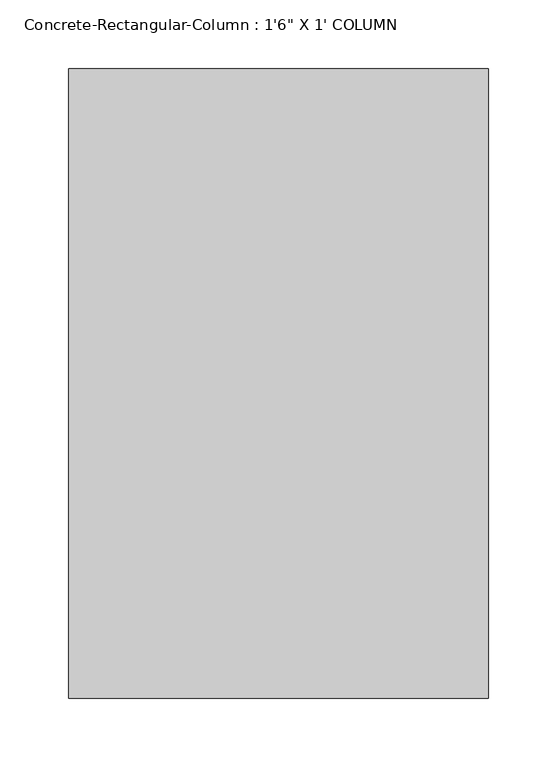
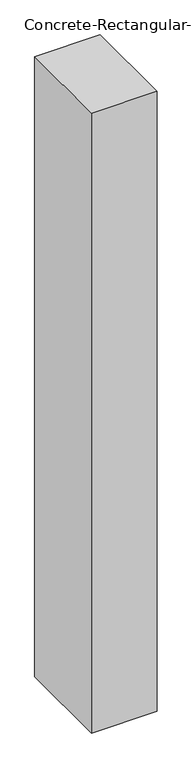
"""IFC4 building model written with IfcOpenShell, lengths in millimetres: column geometry."""

from ifc_helpers import new_model, si_unit, frame, origin, place, context, project, spatial, polyline, outline, extrude, source, transform, mapped, element, save


def column_6a931455(model_context):
    return source(origin(), model_context, "Body", "SweptSolid", [
        extrude(outline(polyline([(152.4, 228.6), (152.4, -228.6), (-152.4, -228.6), (-152.4, 228.6), (152.4, 228.6)])), frame((0.0, 0.0, 304.8), z_axis=(0.0, 0.0, 1.0), x_axis=(1.0, 0.0, 0.0)), (0.0, 0.0, 1.0), 3048.0),
    ])


if __name__ == "__main__":
    model = new_model("IFC4")
    model_context = context("Model", 3, world=origin())
    ifc_project = project(units=[si_unit("LENGTHUNIT", "METRE", prefix="MILLI")], contexts=[model_context])
    site = spatial("IfcSite", under=ifc_project)
    building = spatial("IfcBuilding", under=site)
    placement = place(None, origin())
    column_shape = column_6a931455(model_context)
    element("IfcColumn", 1, ObjectType="Concrete-Rectangular-Column : 1'6\" X 1' COLUMN", at=placement, inside=building, context=model_context, shape_type="MappedRepresentation", body=[
        mapped(column_shape, transform((0.0, 0.0, 0.0), x_axis=(1.0, 0.0, 0.0), y_axis=(0.0, 1.0, 0.0), z_axis=(0.0, 0.0, 1.0))),
    ])
    save(model, "model.ifc")

# Revit data of these elements
# Type "Concrete-Rectangular-Column : 1'6\" X 1' COLUMN"
#   Assembly Code = "B10"
#   b = 1' - 0"
#   h = 1' - 6"
#   Structural Material [instance default] = Concrete, Cast-in-Place gray
# Element 1 (IfcColumn, "Concrete-Rectangular-Column : 1'6\" X 1' COLUMN")
#   Structural Material = WARM BEIGE COLOUR
#   Materials on its faces: "WARM BEIGE COLOUR"
# Materials
#   "Concrete, Cast-in-Place gray": class "Concrete", colour RGB 192 192 192, transparency 0, Description = "Cast-in-place concrete", Cost = 0
#   "WARM BEIGE COLOUR": class "Generic", colour RGB 120 120 120, transparency 0, Cost = 0
